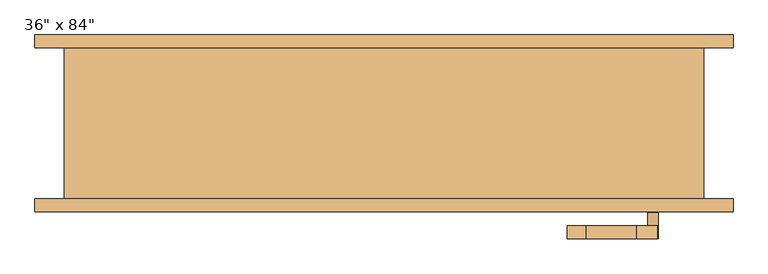
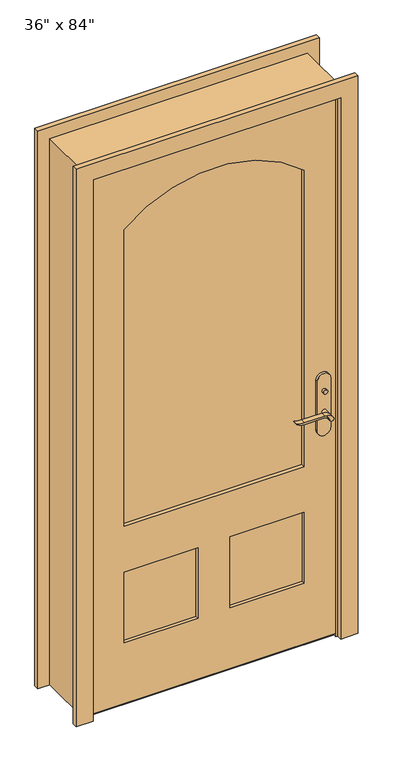
"""IFC4 building model written with IfcOpenShell, lengths in millimetres: door geometry."""

from ifc_helpers import new_model, si_unit, point, frame, frame_2d, origin, place, context, project, spatial, polyline, circle_curve, trimmed, segment, composite_curve, outline, extrude, faceted_brep, source, transform, mapped, element, save


def door_fe8ae985(model_context):
    return source(origin(), model_context, "Body", "SolidModel", [
        extrude(outline(polyline([(-38.1, 12.7), (-12.7, 0.0), (-98.425, 0.0), (-73.025, 12.7), (-38.1, 12.7)])), frame((-457.2, 0.0, 0.0), z_axis=(1.0, 0.0, 0.0), x_axis=(0.0, 1.0, 0.0)), (0.0, 0.0, 1.0), 914.4),
        extrude(outline(polyline([(411.4, -56.2), (411.4, -66.2), (401.4, -66.2), (401.4, -56.2), (411.4, -56.2)])), frame((0.0, 0.0, 981.9), z_axis=(0.0, 0.0, 1.0), x_axis=(1.0, 0.0, 0.0)), (0.0, 0.0, 1.0), 30.0),
        extrude(outline(composite_curve([segment(trimmed(circle_curve(frame_2d((996.9, 406.4)), 8.0), [point((996.9, 398.4))], [point((996.9, 414.4))], False, "CARTESIAN"), True, "CONTINUOUS"), segment(trimmed(circle_curve(frame_2d((996.9, 406.4)), 8.0), [point((996.9, 414.4))], [point((996.9, 398.4))], False, "CARTESIAN"), True, "CONTINUOUS")], self_intersect=False)), frame((0.0, -131.125, 0.0), z_axis=(0.0, 1.0, 0.0), x_axis=(0.0, 0.0, 1.0)), (0.0, 0.0, 1.0), 10.0),
        extrude(outline(composite_curve([segment(trimmed(circle_curve(frame_2d((897.1555521, 382.7324871)), 37.2832219), [point((919.0523287, 412.9081363))], [point((934.4, 381.0325667))], False, "CARTESIAN"), True, "CONTINUOUS"), segment(polyline([(934.4, 381.0325667), (934.4, 304.7564091)]), True, "CONTINUOUS"), segment(trimmed(circle_curve(frame_2d((1017.6850638, 304.8227909)), 83.2850902), [point((934.4, 304.7564091))], [point((939.4, 276.4))], True, "CARTESIAN"), True, "CONTINUOUS"), segment(polyline([(939.4, 276.4), (936.6135558, 276.4)]), True, "CONTINUOUS"), segment(trimmed(circle_curve(frame_2d((986.6709207, 308.3396612)), 59.3791355), [point((936.6135558, 276.4))], [point((927.4, 304.7564091))], False, "CARTESIAN"), True, "CONTINUOUS"), segment(polyline([(927.4, 304.7564091), (927.4, 381.0138099)]), True, "CONTINUOUS"), segment(trimmed(circle_curve(frame_2d((909.2738613, 381.0138099)), 18.1261387), [point((927.4, 381.0138099))], [point((914.4, 398.4))], True, "CARTESIAN"), True, "CONTINUOUS"), segment(trimmed(circle_curve(frame_2d((914.4, 406.4)), 8.0), [point((914.4, 398.4))], [point((919.0523287, 412.9081363))], False, "CARTESIAN"), True, "CONTINUOUS")], self_intersect=False)), frame((0.0, -36.2, 0.0), z_axis=(0.0, 1.0, 0.0), x_axis=(0.0, 0.0, 1.0)), (0.0, 0.0, 1.0), 20.0),
        extrude(outline(composite_curve([segment(trimmed(circle_curve(frame_2d((914.4, 406.4)), 8.0), [point((914.3999903, 398.4))], [point((919.0523287, 412.9081363))], False, "CARTESIAN"), True, "CONTINUOUS"), segment(trimmed(circle_curve(frame_2d((897.1555521, 382.7324871)), 37.2832219), [point((919.0523287, 412.9081363))], [point((934.4, 381.0325667))], False, "CARTESIAN"), True, "CONTINUOUS"), segment(polyline([(934.4, 381.0325667), (934.4, 304.7564091)]), True, "CONTINUOUS"), segment(trimmed(circle_curve(frame_2d((1017.6850638, 304.8227909)), 83.2850902), [point((934.4, 304.7564091))], [point((939.4, 276.4))], True, "CARTESIAN"), True, "CONTINUOUS"), segment(polyline([(939.4, 276.4), (936.6135558, 276.4)]), True, "CONTINUOUS"), segment(trimmed(circle_curve(frame_2d((986.6709207, 308.3396612)), 59.3791355), [point((936.6135558, 276.4))], [point((927.4, 304.7564091))], False, "CARTESIAN"), True, "CONTINUOUS"), segment(polyline([(927.4, 304.7564091), (927.4, 381.0138122)]), True, "CONTINUOUS"), segment(trimmed(circle_curve(frame_2d((909.2738682, 381.0138122)), 18.1261318), [point((927.4, 381.0138122))], [point((914.3999903, 398.4))], True, "CARTESIAN"), True, "CONTINUOUS")], self_intersect=False)), frame((0.0, -171.125, 0.0), z_axis=(0.0, 1.0, 0.0), x_axis=(0.0, 0.0, 1.0)), (0.0, 0.0, 1.0), 20.0),
        extrude(outline(composite_curve([segment(trimmed(circle_curve(frame_2d((914.4, 406.4)), 8.0), [point((914.4, 398.4))], [point((914.4, 414.4))], False, "CARTESIAN"), True, "CONTINUOUS"), segment(trimmed(circle_curve(frame_2d((914.4, 406.4)), 8.0), [point((914.4, 414.4))], [point((914.4, 398.4))], False, "CARTESIAN"), True, "CONTINUOUS")], self_intersect=False)), frame((0.0, -66.2, 0.0), z_axis=(0.0, 1.0, 0.0), x_axis=(0.0, 0.0, 1.0)), (0.0, 0.0, 1.0), 30.0),
        extrude(outline(composite_curve([segment(trimmed(circle_curve(frame_2d((914.4, 406.4)), 8.0), [point((914.4, 398.4))], [point((914.4, 414.4))], False, "CARTESIAN"), True, "CONTINUOUS"), segment(trimmed(circle_curve(frame_2d((914.4, 406.4)), 8.0), [point((914.4, 414.4))], [point((914.4, 398.4))], False, "CARTESIAN"), True, "CONTINUOUS")], self_intersect=False)), frame((0.0, -151.125, 0.0), z_axis=(0.0, 1.0, 0.0), x_axis=(0.0, 0.0, 1.0)), (0.0, 0.0, 1.0), 30.0),
        extrude(outline(composite_curve([segment(polyline([(844.4, 431.4), (1039.4, 431.4)]), True, "CONTINUOUS"), segment(trimmed(circle_curve(frame_2d((1039.4, 406.4)), 25.0), [point((1039.4, 431.4))], [point((1039.4, 381.4))], False, "CARTESIAN"), True, "CONTINUOUS"), segment(polyline([(1039.4, 381.4), (844.4, 381.4)]), True, "CONTINUOUS"), segment(trimmed(circle_curve(frame_2d((844.4, 406.4)), 25.0), [point((844.4, 381.4))], [point((844.4, 431.4))], False, "CARTESIAN"), True, "CONTINUOUS")], self_intersect=False)), frame((0.0, -76.2, 0.0), z_axis=(0.0, 1.0, 0.0), x_axis=(0.0, 0.0, 1.0)), (0.0, 0.0, 1.0), 10.0),
        extrude(outline(composite_curve([segment(polyline([(844.4, 431.4), (1039.4, 431.4)]), True, "CONTINUOUS"), segment(trimmed(circle_curve(frame_2d((1039.4, 406.4)), 25.0), [point((1039.4, 431.4))], [point((1039.4, 381.4))], False, "CARTESIAN"), True, "CONTINUOUS"), segment(polyline([(1039.4, 381.4), (844.4, 381.4)]), True, "CONTINUOUS"), segment(trimmed(circle_curve(frame_2d((844.4, 406.4)), 25.0), [point((844.4, 381.4))], [point((844.4, 431.4))], False, "CARTESIAN"), True, "CONTINUOUS")], self_intersect=False)), frame((0.0, -121.125, 0.0), z_axis=(0.0, 1.0, 0.0), x_axis=(0.0, 0.0, 1.0)), (0.0, 0.0, 1.0), 10.0),
        faceted_brep([(482.6, -111.125, 0.0), (457.2, -111.125, 0.0), (457.2, -76.2, 0.0), (444.5, -76.2, 0.0), (444.5, -41.275, 0.0), (457.2, -41.275, 0.0), (457.2, 117.475, 0.0), (482.6, 117.475, 0.0), (482.6, 117.475, 2159.0), (482.6, -111.125, 2159.0), (457.2, 117.475, 2133.6), (-457.2, 117.475, 2133.6), (-457.2, 117.475, 0.0), (-482.6, 117.475, 0.0), (-482.6, 117.475, 2159.0), (457.2, -41.275, 2133.6), (444.5, -41.275, 2120.9), (-444.5, -41.275, 2120.9), (-444.5, -41.275, 0.0), (-457.2, -41.275, 0.0), (-457.2, -41.275, 2133.6), (444.5, -76.2, 2120.9), (457.2, -76.2, 2133.6), (-457.2, -76.2, 2133.6), (-457.2, -76.2, 0.0), (-444.5, -76.2, 0.0), (-444.5, -76.2, 2120.9), (457.2, -111.125, 2133.6), (-482.6, -111.125, 2159.0), (-482.6, -111.125, 0.0), (-457.2, -111.125, 0.0), (-457.2, -111.125, 2133.6)], [[[0, 1, 2, 3, 4, 5, 6, 7]], [[7, 8, 9, 0]], [[6, 10, 11, 12, 13, 14, 8, 7]], [[5, 15, 10, 6]], [[4, 16, 17, 18, 19, 20, 15, 5]], [[3, 21, 16, 4]], [[2, 22, 23, 24, 25, 26, 21, 3]], [[1, 27, 22, 2]], [[0, 9, 28, 29, 30, 31, 27, 1]], [[8, 14, 28, 9]], [[15, 20, 11, 10]], [[21, 26, 17, 16]], [[27, 31, 23, 22]], [[29, 13, 12, 19, 18, 25, 24, 30]], [[14, 13, 29, 28]], [[20, 19, 12, 11]], [[26, 25, 18, 17]], [[31, 30, 24, 23]]]),
        extrude(outline(polyline([(2133.6, -457.2), (12.7, -457.2), (12.7, 457.2), (2133.6, 457.2), (2133.6, -457.2)]), holes=[composite_curve([segment(polyline([(714.375, -336.55), (1885.95, -336.55)]), True, "CONTINUOUS"), segment(trimmed(circle_curve(frame_2d((1503.52125, 0.0)), 509.42875), [point((1885.95, -336.55))], [point((1885.95, 336.55))], True, "CARTESIAN"), True, "CONTINUOUS"), segment(polyline([(1885.95, 336.55), (714.375, 336.55), (714.375, -336.55)]), True, "CONTINUOUS")], self_intersect=False), polyline([(533.4, -60.325), (254.0, -60.325), (254.0, -336.55), (533.4, -336.55), (533.4, -60.325)]), polyline([(533.4, 336.55), (254.0, 336.55), (254.0, 60.325), (533.4, 60.325), (533.4, 336.55)])]), frame((0.0, -111.125, 0.0), z_axis=(0.0, 1.0, 0.0), x_axis=(0.0, 0.0, 1.0)), (0.0, 0.0, 1.0), 34.925),
        extrude(outline(composite_curve([segment(polyline([(714.375, -336.55), (714.375, 336.55), (1885.95, 336.55)]), True, "CONTINUOUS"), segment(trimmed(circle_curve(frame_2d((1503.52125, 0.0)), 509.42875), [point((1885.95, 336.55))], [point((1885.95, -336.55))], False, "CARTESIAN"), True, "CONTINUOUS"), segment(polyline([(1885.95, -336.55), (714.375, -336.55)]), True, "CONTINUOUS")], self_intersect=False)), frame((0.0, -97.155, 0.0), z_axis=(0.0, 1.0, 0.0), x_axis=(0.0, 0.0, 1.0)), (0.0, 0.0, 1.0), 6.985),
        extrude(outline(polyline([(-60.325, -87.8416667), (-60.325, -99.4833333), (-336.55, -99.4833333), (-336.55, -87.8416667), (-60.325, -87.8416667)])), frame((0.0, 0.0, 254.0), z_axis=(0.0, 0.0, 1.0), x_axis=(1.0, 0.0, 0.0)), (0.0, 0.0, 1.0), 279.4),
        extrude(outline(polyline([(336.55, -87.8416667), (336.55, -99.4833333), (60.325, -99.4833333), (60.325, -87.8416667), (336.55, -87.8416667)])), frame((0.0, 0.0, 254.0), z_axis=(0.0, 0.0, 1.0), x_axis=(1.0, 0.0, 0.0)), (0.0, 0.0, 1.0), 279.4),
        extrude(outline(polyline([(0.0, -463.55), (2139.95, -463.55), (2139.95, 463.55), (0.0, 463.55), (0.0, 527.05), (2203.45, 527.05), (2203.45, -527.05), (0.0, -527.05), (0.0, -463.55)])), frame((0.0, -130.175, 0.0), z_axis=(0.0, 1.0, 0.0), x_axis=(0.0, 0.0, 1.0)), (0.0, 0.0, 1.0), 19.05),
        extrude(outline(polyline([(0.0, -463.55), (2139.95, -463.55), (2139.95, 463.55), (0.0, 463.55), (0.0, 527.05), (2203.45, 527.05), (2203.45, -527.05), (0.0, -527.05), (0.0, -463.55)])), frame((0.0, 117.475, 0.0), z_axis=(0.0, 1.0, 0.0), x_axis=(0.0, 0.0, 1.0)), (0.0, 0.0, 1.0), 19.05),
    ])


if __name__ == "__main__":
    model = new_model("IFC4")
    model_context = context("Model", 3, world=origin())
    ifc_project = project(units=[si_unit("LENGTHUNIT", "METRE", prefix="MILLI")], contexts=[model_context])
    site = spatial("IfcSite", under=ifc_project)
    building = spatial("IfcBuilding", under=site)
    placement = place(None, origin())
    door_shape = door_fe8ae985(model_context)
    element("IfcDoor", 1, ObjectType="36\" x 84\"", at=placement, inside=building, context=model_context, shape_type="MappedRepresentation", body=[
        mapped(door_shape, transform((0.0, 0.0, 0.0), x_axis=(1.0, 0.0, 0.0), y_axis=(0.0, 1.0, 0.0), z_axis=(0.0, 0.0, 1.0))),
    ])
    save(model, "model.ifc")

# Revit data of these elements
# Type "36\" x 84\""
#   Type Mark = "11"
#   Assembly Code = "B2030100"
#   Analytic Construction = "French door, wood frame with single glass"
#   Threshold Offset [instance default] = 0' - 0 1/2"
#   Thickness = 0' - 1 3/8"
#   Thermal Resistance (R) = 1.0696 (h·ft²·°F)/BTU
#   Swing Angle [instance default] = 90.00°
#   Stiles = 0' - 4 3/4"
#   Rough Width = 3' - 2"
#   Rough Height = 7' - 1"
#   Radius = 1' - 8.05625"
#   Lock Rail = 0' - 7 1/8"
#   Height = 7' - 0"
#   Width = 3' - 0"
#   Heat Transfer Coefficient (U) = 0.9350 BTU/(h·ft²·°F)
#   Door Offset [instance default] = 0' - 0"
#   Bottom Rail = 0' - 9 1/2"
#   Threshold [instance default] = yes
#   Function = 1
#   Exterior Trim [instance default] = yes
#   Trim Material = Cherry
#   Threshold Material = Cherry
#   Panel Material = Cherry
#   Glazing = Glass
#   Frame Material = Cherry
#   Door Handle Material = Aluminum
#   Visual Light Transmittance = 0
#   Solar Heat Gain Coefficient = 0
#   Wall Closure = (empty or 0)
#   Construction Type = (empty or 0)
# Element 1 (IfcDoor, "36\" x 84\"")
#   Materials on its faces: "Cherry", "Aluminum", "Glass"
# Materials
#   "Cherry": class "Wood", colour RGB 226 177 128, transparency 0, Description = "Prunus Serotina", Cost = 0
#   "Glass": class "Glass", colour RGB 0 128 192, transparency 0.75, Description = "Soda Lime Glass", Cost = 0
#   "Aluminum": class "Metal", colour RGB 247 247 247, transparency 0, Description = "Aluminum 6061", Cost = 0
